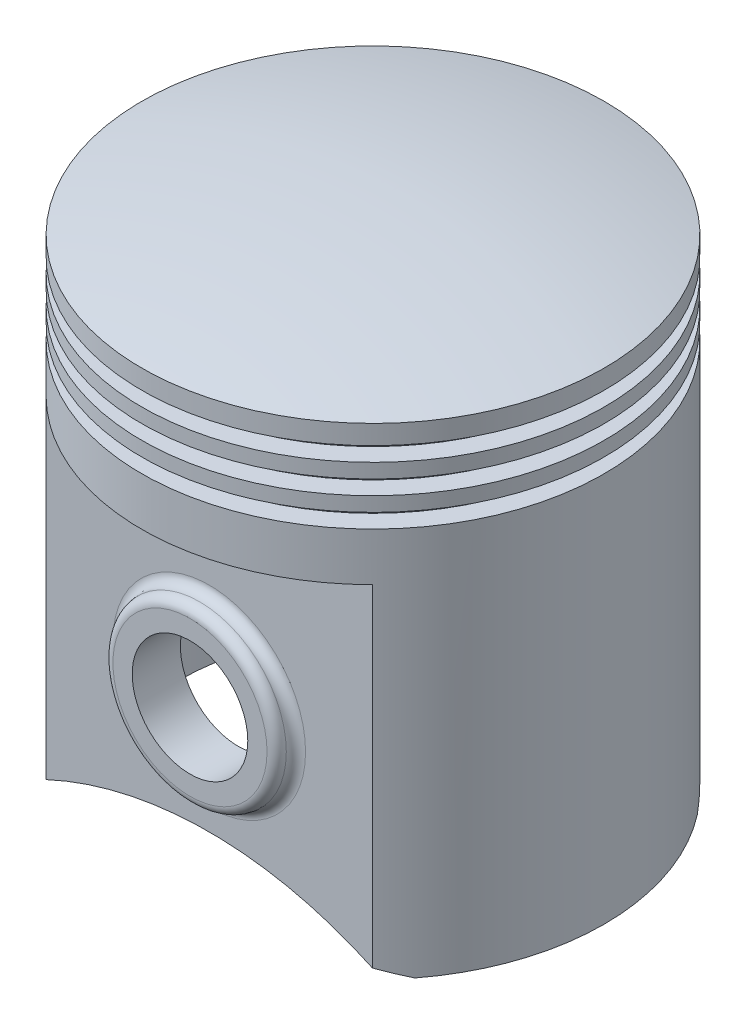
ISO-10303-21;
HEADER;
FILE_DESCRIPTION(('STEP AP214'),'2;1');
FILE_NAME('part.step','',(''),(''),'','','');
FILE_SCHEMA(('AUTOMOTIVE_DESIGN { 1 0 10303 214 1 1 1 1 }'));
ENDSEC;
DATA;
#1=APPLICATION_CONTEXT('core data for automotive mechanical design processes');
#2=APPLICATION_PROTOCOL_DEFINITION('international standard','automotive_design',2000,#1);
#3=PRODUCT_CONTEXT('',#1,'mechanical');
#4=PRODUCT('Part','Part','',(#3));
#5=PRODUCT_RELATED_PRODUCT_CATEGORY('part','',(#4));
#6=PRODUCT_DEFINITION_FORMATION('','',#4);
#7=PRODUCT_DEFINITION_CONTEXT('part definition',#1,'design');
#8=PRODUCT_DEFINITION('design','',#6,#7);
#9=PRODUCT_DEFINITION_SHAPE('','',#8);
#10=(LENGTH_UNIT() NAMED_UNIT(*) SI_UNIT(.MILLI.,.METRE.));
#11=(NAMED_UNIT(*) PLANE_ANGLE_UNIT() SI_UNIT($,.RADIAN.));
#12=(NAMED_UNIT(*) SI_UNIT($,.STERADIAN.) SOLID_ANGLE_UNIT());
#13=UNCERTAINTY_MEASURE_WITH_UNIT(LENGTH_MEASURE(1.E-05),#10,'distance_accuracy_value','');
#14=(GEOMETRIC_REPRESENTATION_CONTEXT(3) GLOBAL_UNCERTAINTY_ASSIGNED_CONTEXT((#13)) GLOBAL_UNIT_ASSIGNED_CONTEXT((#10,
#11,#12)) REPRESENTATION_CONTEXT('',''));
#15=CARTESIAN_POINT('',(0.,0.,0.));
#16=DIRECTION('',(0.,0.,1.));
#17=DIRECTION('',(1.,0.,0.));
#18=AXIS2_PLACEMENT_3D('',#15,#16,#17);
#19=CARTESIAN_POINT('',(0.,-35.1994318135961,-24.));
#20=DIRECTION('',(0.,0.,1.));
#21=DIRECTION('',(1.,0.,0.));
#22=AXIS2_PLACEMENT_3D('',#19,#20,#21);
#23=CYLINDRICAL_SURFACE('',#22,40.);
#24=CARTESIAN_POINT('',(19.,0.,14.6628782986152));
#25=CARTESIAN_POINT('',(18.5847844154625,0.22417514231841,15.2008416674184));
#26=CARTESIAN_POINT('',(18.1472749531916,0.450800853525988,15.720583924078));
#27=CARTESIAN_POINT('',(17.229430924885,0.903305358323858,16.7214980336072));
#28=CARTESIAN_POINT('',(16.7490810754239,1.12918385529891,17.2026560042297));
#29=CARTESIAN_POINT('',(15.7443796223877,1.57581717355902,18.1268646371823));
#30=CARTESIAN_POINT('',(15.2197634518151,1.79652939269345,18.5696486228512));
#31=CARTESIAN_POINT('',(14.1313833599364,2.22577453935094,19.4107434347561));
#32=CARTESIAN_POINT('',(13.5676231295076,2.43430861174211,19.8090584447426));
#33=CARTESIAN_POINT('',(12.4014963081478,2.83455429887705,20.5593059044338));
#34=CARTESIAN_POINT('',(11.7990100002299,3.02620893339201,20.9110831218259));
#35=CARTESIAN_POINT('',(10.5602218766716,3.3868064026951,21.5632002725983));
#36=CARTESIAN_POINT('',(9.92391895773195,3.55574849582937,21.8635385263817));
#37=CARTESIAN_POINT('',(8.62342320840555,3.86566866892299,22.4083047027535));
#38=CARTESIAN_POINT('',(7.95931483522713,4.00672490493522,22.6528891907548));
#39=CARTESIAN_POINT('',(6.60663592930378,4.25719223749272,23.0836725338871));
#40=CARTESIAN_POINT('',(5.91806903944259,4.36660802460178,23.2698800435048));
#41=CARTESIAN_POINT('',(4.59215338262825,4.54114914570338,23.5653660010413));
#42=CARTESIAN_POINT('',(3.95653429291983,4.60960046747166,23.6804595182362));
#43=CARTESIAN_POINT('',(2.67557620841154,4.71615638306671,23.8591567014349));
#44=CARTESIAN_POINT('',(2.03023785659978,4.75426297547383,23.9227637584713));
#45=CARTESIAN_POINT('',(0.735406969306551,4.79905416078167,23.9974950965044));
#46=CARTESIAN_POINT('',(0.0859142139936218,4.80573707688299,24.0086165768174));
#47=CARTESIAN_POINT('',(-1.21136844174268,4.78748235913691,23.9781873674946));
#48=CARTESIAN_POINT('',(-1.85915844199787,4.76254662247324,23.9366398381071));
#49=CARTESIAN_POINT('',(-3.08243340113651,4.68584919285358,23.8083586990923));
#50=CARTESIAN_POINT('',(-3.65863458605366,4.63703953335834,23.7265929391012));
#51=CARTESIAN_POINT('',(-4.80109464708866,4.51554548314267,23.5220364728596));
#52=CARTESIAN_POINT('',(-5.36735434428124,4.44286307395504,23.3992491715449));
#53=CARTESIAN_POINT('',(-6.48634583000771,4.27521075369698,23.114080016908));
#54=CARTESIAN_POINT('',(-7.03907894850286,4.18024304356482,22.9517020735703));
#55=CARTESIAN_POINT('',(-8.12798429480032,3.96998748429119,22.5890510227209));
#56=CARTESIAN_POINT('',(-8.66415582672125,3.85469878266769,22.3887763253839));
#57=CARTESIAN_POINT('',(-9.73722129991614,3.60136511760673,21.943940565358));
#58=CARTESIAN_POINT('',(-10.27337378466,3.46262375974749,21.6979896936735));
#59=CARTESIAN_POINT('',(-11.3225328531231,3.16848610713638,21.1694433586757));
#60=CARTESIAN_POINT('',(-11.8355382041687,3.01308892688204,20.8868459468909));
#61=CARTESIAN_POINT('',(-12.8366727755807,2.68852054240194,20.2869564707954));
#62=CARTESIAN_POINT('',(-13.3247872626694,2.51934133079035,19.9696441998403));
#63=CARTESIAN_POINT('',(-14.2741592843496,2.17039703659009,19.3024597608394));
#64=CARTESIAN_POINT('',(-14.7354193578949,1.9906329579918,18.9525906790344));
#65=CARTESIAN_POINT('',(-15.53843000618,1.66118701859229,18.2966765814725));
#66=CARTESIAN_POINT('',(-15.8853582872057,1.51285349768682,17.9962608691975));
#67=CARTESIAN_POINT('',(-16.5607191727584,1.21319010561359,17.376780524918));
#68=CARTESIAN_POINT('',(-16.8891537602792,1.06186055805686,17.0577178998414));
#69=CARTESIAN_POINT('',(-17.5260491906291,0.758343983174592,16.4026139472068));
#70=CARTESIAN_POINT('',(-17.8345646435942,0.606160662421761,16.0666239670156));
#71=CARTESIAN_POINT('',(-18.4320760770373,0.302273870423554,15.377465633861));
#72=CARTESIAN_POINT('',(-18.7210707877824,0.150570431002778,15.0242961660177));
#73=CARTESIAN_POINT('',(-19.,0.,14.6628782986152));
#74=B_SPLINE_CURVE_WITH_KNOTS('',3,(#24,#25,#26,#27,#28,#29,#30,#31,#32,#33,#34,#35,#36,#37,#38,
#39,#40,#41,#42,#43,#44,#45,#46,#47,#48,#49,#50,#51,#52,#53,#54,#55,#56,#57,#58,#59,#60,#61,#62,
#63,#64,#65,#66,#67,#68,#69,#70,#71,#72,#73),.UNSPECIFIED.,.F.,.F.,(4,2,2,2,2,2,2,2,2,2,2,2,2,2,
2,2,2,2,2,2,2,2,2,2,4),(0.,2.14619201814741,4.29315278252665,6.45400344697563,8.6146506416545,
10.7823323717961,12.9500848680932,15.1116728494894,17.2729402200685,19.218937601111,
21.1648068032574,23.1107798377901,25.0566361154919,26.8066791459319,28.5565769525621,
30.3063020086725,32.0561004846409,33.872158160539,35.6883124346079,37.5055295280586,
39.3225745325596,40.7687722984554,42.2148146987619,43.6567076951116,45.0986943897096),.UNSPECIFIED.);
#75=CARTESIAN_POINT('',(19.,0.,14.6628782986152));
#76=VERTEX_POINT('',#75);
#77=CARTESIAN_POINT('',(16.9410743460974,1.03591005039079,17.));
#78=VERTEX_POINT('',#77);
#79=EDGE_CURVE('E202',#76,#78,#74,.T.);
#80=ORIENTED_EDGE('',*,*,#79,.T.);
#81=CARTESIAN_POINT('',(0.,-35.1994318135961,17.));
#82=DIRECTION('',(0.,0.,-1.));
#83=DIRECTION('',(-1.,0.,0.));
#84=AXIS2_PLACEMENT_3D('',#81,#82,#83);
#85=CIRCLE('',#84,40.);
#86=CARTESIAN_POINT('',(-16.9410743460974,1.03591005039079,17.));
#87=VERTEX_POINT('',#86);
#88=EDGE_CURVE('E154',#78,#87,#85,.F.);
#89=ORIENTED_EDGE('',*,*,#88,.T.);
#90=CARTESIAN_POINT('',(-19.,0.,14.6628782986152));
#91=VERTEX_POINT('',#90);
#92=EDGE_CURVE('E153',#87,#91,#74,.T.);
#93=ORIENTED_EDGE('',*,*,#92,.T.);
#94=DIRECTION('',(0.,0.,1.));
#95=VECTOR('',#94,1.);
#96=CARTESIAN_POINT('',(-19.,0.,-24.));
#97=LINE('',#96,#95);
#98=CARTESIAN_POINT('',(-19.,0.,6.24499799839839));
#99=VERTEX_POINT('',#98);
#100=EDGE_CURVE('E291',#91,#99,#97,.F.);
#101=ORIENTED_EDGE('',*,*,#100,.T.);
#102=CARTESIAN_POINT('',(-19.,0.,6.24499799839837));
#103=CARTESIAN_POINT('',(-18.8202585353319,0.0969817128532858,6.79197210301841));
#104=CARTESIAN_POINT('',(-18.6174589709661,0.204714498288521,7.32924799218901));
#105=CARTESIAN_POINT('',(-18.1681410350363,0.437393377984401,8.38124634634524));
#106=CARTESIAN_POINT('',(-17.9216299338799,0.562336608913622,8.89597254422526));
#107=CARTESIAN_POINT('',(-17.3921059919807,0.822781911629741,9.89072900060968));
#108=CARTESIAN_POINT('',(-17.1098421840393,0.958049413971564,10.3712212939202));
#109=CARTESIAN_POINT('',(-16.5076269288855,1.23692809207039,11.3051661022802));
#110=CARTESIAN_POINT('',(-16.1876897852406,1.38053609073414,11.7586287818938));
#111=CARTESIAN_POINT('',(-15.6075875463034,1.63089351304631,12.5124400289307));
#112=CARTESIAN_POINT('',(-15.3560767786114,1.73659212557669,12.8198482567428));
#113=CARTESIAN_POINT('',(-14.8336181639409,1.94951117012887,13.4210039659551));
#114=CARTESIAN_POINT('',(-14.5625515542914,2.05673705236659,13.7146463148781));
#115=CARTESIAN_POINT('',(-14.2828568570857,2.16365157094273,14.));
#116=B_SPLINE_CURVE_WITH_KNOTS('',3,(#102,#103,#104,#105,#106,#107,#108,#109,#110,#111,#112,
#113,#114,#115),.UNSPECIFIED.,.F.,.F.,(4,2,2,2,2,2,4),(0.,1.75066829987974,3.50104568906382,
5.21944897719957,6.93720192412629,8.16959104224677,9.41022371268353),.UNSPECIFIED.);
#117=CARTESIAN_POINT('',(-14.2828568570857,2.16365157094273,14.));
#118=VERTEX_POINT('',#117);
#119=EDGE_CURVE('E413',#99,#118,#116,.T.);
#120=ORIENTED_EDGE('',*,*,#119,.T.);
#121=CARTESIAN_POINT('',(0.,-35.1994318135961,14.));
#122=DIRECTION('',(0.,0.,1.));
#123=DIRECTION('',(1.,0.,0.));
#124=AXIS2_PLACEMENT_3D('',#121,#122,#123);
#125=CIRCLE('',#124,40.);
#126=CARTESIAN_POINT('',(14.2828568570857,2.16365157094272,14.));
#127=VERTEX_POINT('',#126);
#128=EDGE_CURVE('E253',#118,#127,#125,.F.);
#129=ORIENTED_EDGE('',*,*,#128,.T.);
#130=CARTESIAN_POINT('',(14.2828568570857,2.16365157094272,14.));
#131=CARTESIAN_POINT('',(14.6775131687569,2.01280729699775,13.5973677537348));
#132=CARTESIAN_POINT('',(15.0550498418311,1.8612961791732,13.1781481636073));
#133=CARTESIAN_POINT('',(15.7741579232714,1.56097502677152,12.3083178308759));
#134=CARTESIAN_POINT('',(16.1156954030899,1.41216764779983,11.857678128264));
#135=CARTESIAN_POINT('',(16.7541220935511,1.12438631173865,10.9365144759754));
#136=CARTESIAN_POINT('',(17.0517449304083,0.98527811151048,10.4665411255795));
#137=CARTESIAN_POINT('',(17.6077757822892,0.717991544973343,9.50137374432842));
#138=CARTESIAN_POINT('',(17.8662123403,0.589805253334924,9.00619842497101));
#139=CARTESIAN_POINT('',(18.2746614216328,0.38249383567688,8.13621217368548));
#140=CARTESIAN_POINT('',(18.4346757038592,0.299740972735459,7.76692986093451));
#141=CARTESIAN_POINT('',(18.7337473919056,0.14282623615124,7.01509751919342));
#142=CARTESIAN_POINT('',(18.8726505382507,0.0687284369135807,6.63247280860509));
#143=CARTESIAN_POINT('',(19.,0.,6.2449979983984));
#144=B_SPLINE_CURVE_WITH_KNOTS('',3,(#130,#131,#132,#133,#134,#135,#136,#137,#138,#139,#140,
#141,#142,#143),.UNSPECIFIED.,.F.,.F.,(4,2,2,2,2,2,4),(0.,1.75046610713076,3.50256751449379,
5.22090157760208,6.93797794376393,8.1698351473774,9.41030051506601),.UNSPECIFIED.);
#145=CARTESIAN_POINT('',(19.,0.,6.2449979983984));
#146=VERTEX_POINT('',#145);
#147=EDGE_CURVE('E241',#127,#146,#144,.T.);
#148=ORIENTED_EDGE('',*,*,#147,.T.);
#149=DIRECTION('',(0.,0.,1.));
#150=VECTOR('',#149,1.);
#151=CARTESIAN_POINT('',(19.,0.,-24.));
#152=LINE('',#151,#150);
#153=EDGE_CURVE('E281',#146,#76,#152,.T.);
#154=ORIENTED_EDGE('',*,*,#153,.T.);
#155=EDGE_LOOP('',(#80,#89,#93,#101,#120,#129,#148,#154));
#156=FACE_BOUND('',#155,.T.);
#157=ADVANCED_FACE('F44',(#156),#23,.F.);
#158=CARTESIAN_POINT('',(0.,0.,0.));
#159=DIRECTION('',(0.,-1.,0.));
#160=DIRECTION('',(0.,0.,-1.));
#161=AXIS2_PLACEMENT_3D('',#158,#159,#160);
#162=PLANE('',#161);
#163=CARTESIAN_POINT('',(0.,0.,0.));
#164=DIRECTION('',(0.,-1.,0.));
#165=DIRECTION('',(0.,0.,-1.));
#166=AXIS2_PLACEMENT_3D('',#163,#164,#165);
#167=CIRCLE('',#166,20.);
#168=CARTESIAN_POINT('',(19.,0.,-6.2449979983984));
#169=VERTEX_POINT('',#168);
#170=EDGE_CURVE('E175',#169,#146,#167,.T.);
#171=ORIENTED_EDGE('',*,*,#170,.F.);
#172=CARTESIAN_POINT('',(19.,0.,-14.6628782986152));
#173=VERTEX_POINT('',#172);
#174=EDGE_CURVE('E315',#173,#169,#152,.T.);
#175=ORIENTED_EDGE('',*,*,#174,.F.);
#176=CARTESIAN_POINT('',(0.,0.,0.));
#177=DIRECTION('',(0.,-1.,0.));
#178=DIRECTION('',(0.,0.,-1.));
#179=AXIS2_PLACEMENT_3D('',#176,#177,#178);
#180=CIRCLE('',#179,24.);
#181=EDGE_CURVE('E289',#173,#76,#180,.T.);
#182=ORIENTED_EDGE('',*,*,#181,.T.);
#183=ORIENTED_EDGE('',*,*,#153,.F.);
#184=EDGE_LOOP('',(#171,#175,#182,#183));
#185=FACE_BOUND('',#184,.T.);
#186=ADVANCED_FACE('F275',(#185),#162,.T.);
#187=CARTESIAN_POINT('',(0.,-43.9999798630667,-0.0625025171167009));
#188=DIRECTION('',(-1.,0.,0.));
#189=DIRECTION('',(0.,0.,-1.));
#190=AXIS2_PLACEMENT_3D('',#187,#188,#189);
#191=CIRCLE('',#190,97.);
#192=TRIMMED_CURVE('',#191,(PARAMETER_VALUE(-1.57144068268605)),
(PARAMETER_VALUE(1.57144068268605)),.T.,.PARAMETER.);
#193=CARTESIAN_POINT('',(0.,-43.9999798630667,0.));
#194=DIRECTION('',(0.,-1.,0.));
#195=AXIS1_PLACEMENT('',#193,#194);
#196=SURFACE_OF_REVOLUTION('',#192,#195);
#197=CARTESIAN_POINT('',(0.,53.,0.));
#198=VERTEX_POINT('',#197);
#199=VERTEX_LOOP('',#198);
#200=FACE_BOUND('',#199,.T.);
#201=CARTESIAN_POINT('',(0.,50.,0.));
#202=DIRECTION('',(0.,-1.,0.));
#203=DIRECTION('',(0.,0.,-1.));
#204=AXIS2_PLACEMENT_3D('',#201,#202,#203);
#205=CIRCLE('',#204,24.);
#206=CARTESIAN_POINT('',(0.,50.,-24.));
#207=VERTEX_POINT('',#206);
#208=EDGE_CURVE('E308',#207,#207,#205,.T.);
#209=ORIENTED_EDGE('',*,*,#208,.F.);
#210=EDGE_LOOP('',(#209));
#211=FACE_BOUND('',#210,.T.);
#212=ADVANCED_FACE('F276',(#200,#211),#196,.T.);
#213=CARTESIAN_POINT('',(0.,0.,0.));
#214=DIRECTION('',(0.,-1.,0.));
#215=DIRECTION('',(0.,0.,-1.));
#216=AXIS2_PLACEMENT_3D('',#213,#214,#215);
#217=CYLINDRICAL_SURFACE('',#216,24.);
#218=ORIENTED_EDGE('',*,*,#208,.T.);
#219=EDGE_LOOP('',(#218));
#220=FACE_BOUND('',#219,.T.);
#221=CARTESIAN_POINT('',(0.,48.,0.));
#222=DIRECTION('',(0.,-1.,0.));
#223=DIRECTION('',(0.,0.,-1.));
#224=AXIS2_PLACEMENT_3D('',#221,#222,#223);
#225=CIRCLE('',#224,24.);
#226=CARTESIAN_POINT('',(0.,48.,-24.));
#227=VERTEX_POINT('',#226);
#228=EDGE_CURVE('E306',#227,#227,#225,.T.);
#229=ORIENTED_EDGE('',*,*,#228,.F.);
#230=EDGE_LOOP('',(#229));
#231=FACE_BOUND('',#230,.T.);
#232=ADVANCED_FACE('F356',(#220,#231),#217,.T.);
#233=CARTESIAN_POINT('',(22.,48.,0.));
#234=DIRECTION('',(0.,-1.,0.));
#235=DIRECTION('',(0.,0.,-1.));
#236=AXIS2_PLACEMENT_3D('',#233,#234,#235);
#237=PLANE('',#236);
#238=ORIENTED_EDGE('',*,*,#228,.T.);
#239=EDGE_LOOP('',(#238));
#240=FACE_BOUND('',#239,.T.);
#241=CARTESIAN_POINT('',(0.,48.,0.));
#242=DIRECTION('',(0.,-1.,0.));
#243=DIRECTION('',(0.,0.,-1.));
#244=AXIS2_PLACEMENT_3D('',#241,#242,#243);
#245=CIRCLE('',#244,22.);
#246=CARTESIAN_POINT('',(0.,48.,-22.));
#247=VERTEX_POINT('',#246);
#248=EDGE_CURVE('E348',#247,#247,#245,.T.);
#249=ORIENTED_EDGE('',*,*,#248,.F.);
#250=EDGE_LOOP('',(#249));
#251=FACE_BOUND('',#250,.T.);
#252=ADVANCED_FACE('F353',(#240,#251),#237,.T.);
#253=CARTESIAN_POINT('',(0.,0.,0.));
#254=DIRECTION('',(0.,-1.,0.));
#255=DIRECTION('',(0.,0.,-1.));
#256=AXIS2_PLACEMENT_3D('',#253,#254,#255);
#257=CYLINDRICAL_SURFACE('',#256,22.);
#258=ORIENTED_EDGE('',*,*,#248,.T.);
#259=EDGE_LOOP('',(#258));
#260=FACE_BOUND('',#259,.T.);
#261=CARTESIAN_POINT('',(0.,46.5,0.));
#262=DIRECTION('',(0.,-1.,0.));
#263=DIRECTION('',(0.,0.,-1.));
#264=AXIS2_PLACEMENT_3D('',#261,#262,#263);
#265=CIRCLE('',#264,22.);
#266=CARTESIAN_POINT('',(0.,46.5,-22.));
#267=VERTEX_POINT('',#266);
#268=EDGE_CURVE('E350',#267,#267,#265,.T.);
#269=ORIENTED_EDGE('',*,*,#268,.F.);
#270=EDGE_LOOP('',(#269));
#271=FACE_BOUND('',#270,.T.);
#272=ADVANCED_FACE('F368',(#260,#271),#257,.T.);
#273=CARTESIAN_POINT('',(24.,46.5,0.));
#274=DIRECTION('',(0.,1.,0.));
#275=DIRECTION('',(0.,0.,1.));
#276=AXIS2_PLACEMENT_3D('',#273,#274,#275);
#277=PLANE('',#276);
#278=ORIENTED_EDGE('',*,*,#268,.T.);
#279=EDGE_LOOP('',(#278));
#280=FACE_BOUND('',#279,.T.);
#281=CARTESIAN_POINT('',(0.,46.5,0.));
#282=DIRECTION('',(0.,-1.,0.));
#283=DIRECTION('',(0.,0.,-1.));
#284=AXIS2_PLACEMENT_3D('',#281,#282,#283);
#285=CIRCLE('',#284,24.);
#286=CARTESIAN_POINT('',(0.,46.5,-24.));
#287=VERTEX_POINT('',#286);
#288=EDGE_CURVE('E344',#287,#287,#285,.T.);
#289=ORIENTED_EDGE('',*,*,#288,.F.);
#290=EDGE_LOOP('',(#289));
#291=FACE_BOUND('',#290,.T.);
#292=ADVANCED_FACE('F677',(#280,#291),#277,.T.);
#293=CARTESIAN_POINT('',(0.,0.,0.));
#294=DIRECTION('',(0.,-1.,0.));
#295=DIRECTION('',(0.,0.,-1.));
#296=AXIS2_PLACEMENT_3D('',#293,#294,#295);
#297=CYLINDRICAL_SURFACE('',#296,24.);
#298=ORIENTED_EDGE('',*,*,#288,.T.);
#299=EDGE_LOOP('',(#298));
#300=FACE_BOUND('',#299,.T.);
#301=CARTESIAN_POINT('',(0.,45.,0.));
#302=DIRECTION('',(0.,-1.,0.));
#303=DIRECTION('',(0.,0.,-1.));
#304=AXIS2_PLACEMENT_3D('',#301,#302,#303);
#305=CIRCLE('',#304,24.);
#306=CARTESIAN_POINT('',(0.,45.,-24.));
#307=VERTEX_POINT('',#306);
#308=EDGE_CURVE('E343',#307,#307,#305,.T.);
#309=ORIENTED_EDGE('',*,*,#308,.F.);
#310=EDGE_LOOP('',(#309));
#311=FACE_BOUND('',#310,.T.);
#312=ADVANCED_FACE('F669',(#300,#311),#297,.T.);
#313=CARTESIAN_POINT('',(22.,45.,0.));
#314=DIRECTION('',(0.,-1.,0.));
#315=DIRECTION('',(0.,0.,-1.));
#316=AXIS2_PLACEMENT_3D('',#313,#314,#315);
#317=PLANE('',#316);
#318=ORIENTED_EDGE('',*,*,#308,.T.);
#319=EDGE_LOOP('',(#318));
#320=FACE_BOUND('',#319,.T.);
#321=CARTESIAN_POINT('',(0.,45.,0.));
#322=DIRECTION('',(0.,-1.,0.));
#323=DIRECTION('',(0.,0.,-1.));
#324=AXIS2_PLACEMENT_3D('',#321,#322,#323);
#325=CIRCLE('',#324,22.);
#326=CARTESIAN_POINT('',(0.,45.,-22.));
#327=VERTEX_POINT('',#326);
#328=EDGE_CURVE('E340',#327,#327,#325,.T.);
#329=ORIENTED_EDGE('',*,*,#328,.F.);
#330=EDGE_LOOP('',(#329));
#331=FACE_BOUND('',#330,.T.);
#332=ADVANCED_FACE('F660',(#320,#331),#317,.T.);
#333=CARTESIAN_POINT('',(0.,0.,0.));
#334=DIRECTION('',(0.,-1.,0.));
#335=DIRECTION('',(0.,0.,-1.));
#336=AXIS2_PLACEMENT_3D('',#333,#334,#335);
#337=CYLINDRICAL_SURFACE('',#336,22.);
#338=ORIENTED_EDGE('',*,*,#328,.T.);
#339=EDGE_LOOP('',(#338));
#340=FACE_BOUND('',#339,.T.);
#341=CARTESIAN_POINT('',(0.,43.5,0.));
#342=DIRECTION('',(0.,-1.,0.));
#343=DIRECTION('',(0.,0.,-1.));
#344=AXIS2_PLACEMENT_3D('',#341,#342,#343);
#345=CIRCLE('',#344,22.);
#346=CARTESIAN_POINT('',(0.,43.5,-22.));
#347=VERTEX_POINT('',#346);
#348=EDGE_CURVE('E333',#347,#347,#345,.T.);
#349=ORIENTED_EDGE('',*,*,#348,.F.);
#350=EDGE_LOOP('',(#349));
#351=FACE_BOUND('',#350,.T.);
#352=ADVANCED_FACE('F648',(#340,#351),#337,.T.);
#353=CARTESIAN_POINT('',(24.,43.5,0.));
#354=DIRECTION('',(0.,1.,0.));
#355=DIRECTION('',(0.,0.,1.));
#356=AXIS2_PLACEMENT_3D('',#353,#354,#355);
#357=PLANE('',#356);
#358=ORIENTED_EDGE('',*,*,#348,.T.);
#359=EDGE_LOOP('',(#358));
#360=FACE_BOUND('',#359,.T.);
#361=CARTESIAN_POINT('',(0.,43.5,0.));
#362=DIRECTION('',(0.,-1.,0.));
#363=DIRECTION('',(0.,0.,-1.));
#364=AXIS2_PLACEMENT_3D('',#361,#362,#363);
#365=CIRCLE('',#364,24.);
#366=CARTESIAN_POINT('',(0.,43.5,-24.));
#367=VERTEX_POINT('',#366);
#368=EDGE_CURVE('E335',#367,#367,#365,.T.);
#369=ORIENTED_EDGE('',*,*,#368,.F.);
#370=EDGE_LOOP('',(#369));
#371=FACE_BOUND('',#370,.T.);
#372=ADVANCED_FACE('F640',(#360,#371),#357,.T.);
#373=CARTESIAN_POINT('',(0.,0.,0.));
#374=DIRECTION('',(0.,-1.,0.));
#375=DIRECTION('',(0.,0.,-1.));
#376=AXIS2_PLACEMENT_3D('',#373,#374,#375);
#377=CYLINDRICAL_SURFACE('',#376,24.);
#378=ORIENTED_EDGE('',*,*,#368,.T.);
#379=EDGE_LOOP('',(#378));
#380=FACE_BOUND('',#379,.T.);
#381=CARTESIAN_POINT('',(0.,42.,0.));
#382=DIRECTION('',(0.,-1.,0.));
#383=DIRECTION('',(0.,0.,-1.));
#384=AXIS2_PLACEMENT_3D('',#381,#382,#383);
#385=CIRCLE('',#384,24.);
#386=CARTESIAN_POINT('',(0.,42.,-24.));
#387=VERTEX_POINT('',#386);
#388=EDGE_CURVE('E328',#387,#387,#385,.T.);
#389=ORIENTED_EDGE('',*,*,#388,.F.);
#390=EDGE_LOOP('',(#389));
#391=FACE_BOUND('',#390,.T.);
#392=ADVANCED_FACE('F628',(#380,#391),#377,.T.);
#393=CARTESIAN_POINT('',(22.,42.,0.));
#394=DIRECTION('',(0.,-1.,0.));
#395=DIRECTION('',(0.,0.,-1.));
#396=AXIS2_PLACEMENT_3D('',#393,#394,#395);
#397=PLANE('',#396);
#398=ORIENTED_EDGE('',*,*,#388,.T.);
#399=EDGE_LOOP('',(#398));
#400=FACE_BOUND('',#399,.T.);
#401=CARTESIAN_POINT('',(0.,42.,0.));
#402=DIRECTION('',(0.,-1.,0.));
#403=DIRECTION('',(0.,0.,-1.));
#404=AXIS2_PLACEMENT_3D('',#401,#402,#403);
#405=CIRCLE('',#404,22.);
#406=CARTESIAN_POINT('',(0.,42.,-22.));
#407=VERTEX_POINT('',#406);
#408=EDGE_CURVE('E326',#407,#407,#405,.T.);
#409=ORIENTED_EDGE('',*,*,#408,.F.);
#410=EDGE_LOOP('',(#409));
#411=FACE_BOUND('',#410,.T.);
#412=ADVANCED_FACE('F617',(#400,#411),#397,.T.);
#413=CARTESIAN_POINT('',(0.,0.,0.));
#414=DIRECTION('',(0.,-1.,0.));
#415=DIRECTION('',(0.,0.,-1.));
#416=AXIS2_PLACEMENT_3D('',#413,#414,#415);
#417=CYLINDRICAL_SURFACE('',#416,22.);
#418=ORIENTED_EDGE('',*,*,#408,.T.);
#419=EDGE_LOOP('',(#418));
#420=FACE_BOUND('',#419,.T.);
#421=CARTESIAN_POINT('',(0.,40.5,0.));
#422=DIRECTION('',(0.,-1.,0.));
#423=DIRECTION('',(0.,0.,-1.));
#424=AXIS2_PLACEMENT_3D('',#421,#422,#423);
#425=CIRCLE('',#424,22.);
#426=CARTESIAN_POINT('',(0.,40.5,-22.));
#427=VERTEX_POINT('',#426);
#428=EDGE_CURVE('E321',#427,#427,#425,.T.);
#429=ORIENTED_EDGE('',*,*,#428,.F.);
#430=EDGE_LOOP('',(#429));
#431=FACE_BOUND('',#430,.T.);
#432=ADVANCED_FACE('F615',(#420,#431),#417,.T.);
#433=CARTESIAN_POINT('',(24.,40.5,0.));
#434=DIRECTION('',(0.,1.,0.));
#435=DIRECTION('',(0.,0.,1.));
#436=AXIS2_PLACEMENT_3D('',#433,#434,#435);
#437=PLANE('',#436);
#438=ORIENTED_EDGE('',*,*,#428,.T.);
#439=EDGE_LOOP('',(#438));
#440=FACE_BOUND('',#439,.T.);
#441=CARTESIAN_POINT('',(0.,40.5,0.));
#442=DIRECTION('',(0.,-1.,0.));
#443=DIRECTION('',(0.,0.,-1.));
#444=AXIS2_PLACEMENT_3D('',#441,#442,#443);
#445=CIRCLE('',#444,24.);
#446=CARTESIAN_POINT('',(0.,40.5,-24.));
#447=VERTEX_POINT('',#446);
#448=EDGE_CURVE('E317',#447,#447,#445,.T.);
#449=ORIENTED_EDGE('',*,*,#448,.F.);
#450=EDGE_LOOP('',(#449));
#451=FACE_BOUND('',#450,.T.);
#452=ADVANCED_FACE('F610',(#440,#451),#437,.T.);
#453=CARTESIAN_POINT('',(0.,0.,0.));
#454=DIRECTION('',(0.,-1.,0.));
#455=DIRECTION('',(0.,0.,-1.));
#456=AXIS2_PLACEMENT_3D('',#453,#454,#455);
#457=CYLINDRICAL_SURFACE('',#456,24.);
#458=DIRECTION('',(0.,-1.,0.));
#459=VECTOR('',#458,1.);
#460=CARTESIAN_POINT('',(16.9410743460974,35.5,17.));
#461=LINE('',#460,#459);
#462=CARTESIAN_POINT('',(16.9410743460974,35.5,17.));
#463=VERTEX_POINT('',#462);
#464=EDGE_CURVE('E150',#463,#78,#461,.T.);
#465=ORIENTED_EDGE('',*,*,#464,.T.);
#466=ORIENTED_EDGE('',*,*,#79,.F.);
#467=ORIENTED_EDGE('',*,*,#181,.F.);
#468=CARTESIAN_POINT('',(-19.,0.,-14.6628782986152));
#469=CARTESIAN_POINT('',(-18.5847844154625,0.22417514231841,-15.2008416674184));
#470=CARTESIAN_POINT('',(-18.1472749531916,0.450800853525988,-15.720583924078));
#471=CARTESIAN_POINT('',(-17.229430924885,0.903305358323858,-16.7214980336072));
#472=CARTESIAN_POINT('',(-16.7490810754239,1.12918385529891,-17.2026560042297));
#473=CARTESIAN_POINT('',(-15.7443796223877,1.57581717355902,-18.1268646371823));
#474=CARTESIAN_POINT('',(-15.2197634518151,1.79652939269345,-18.5696486228512));
#475=CARTESIAN_POINT('',(-14.1313833599364,2.22577453935094,-19.4107434347561));
#476=CARTESIAN_POINT('',(-13.5676231295076,2.43430861174211,-19.8090584447426));
#477=CARTESIAN_POINT('',(-12.4014963081478,2.83455429887705,-20.5593059044338));
#478=CARTESIAN_POINT('',(-11.7990100002299,3.02620893339201,-20.9110831218259));
#479=CARTESIAN_POINT('',(-10.5602218766716,3.3868064026951,-21.5632002725983));
#480=CARTESIAN_POINT('',(-9.92391895773195,3.55574849582937,-21.8635385263817));
#481=CARTESIAN_POINT('',(-8.62342320840555,3.86566866892299,-22.4083047027535));
#482=CARTESIAN_POINT('',(-7.95931483522713,4.00672490493522,-22.6528891907548));
#483=CARTESIAN_POINT('',(-6.60663592930378,4.25719223749272,-23.0836725338871));
#484=CARTESIAN_POINT('',(-5.91806903944259,4.36660802460178,-23.2698800435048));
#485=CARTESIAN_POINT('',(-4.59215338262825,4.54114914570338,-23.5653660010413));
#486=CARTESIAN_POINT('',(-3.95653429291983,4.60960046747166,-23.6804595182362));
#487=CARTESIAN_POINT('',(-2.67557620841154,4.71615638306671,-23.8591567014349));
#488=CARTESIAN_POINT('',(-2.03023785659978,4.75426297547383,-23.9227637584713));
#489=CARTESIAN_POINT('',(-0.735406969306551,4.79905416078167,-23.9974950965044));
#490=CARTESIAN_POINT('',(-0.0859142139936218,4.80573707688299,-24.0086165768174));
#491=CARTESIAN_POINT('',(1.21136844174268,4.78748235913691,-23.9781873674946));
#492=CARTESIAN_POINT('',(1.85915844199787,4.76254662247324,-23.9366398381071));
#493=CARTESIAN_POINT('',(3.08243340113651,4.68584919285358,-23.8083586990923));
#494=CARTESIAN_POINT('',(3.65863458605366,4.63703953335834,-23.7265929391012));
#495=CARTESIAN_POINT('',(4.80109464708866,4.51554548314267,-23.5220364728596));
#496=CARTESIAN_POINT('',(5.36735434428124,4.44286307395504,-23.3992491715449));
#497=CARTESIAN_POINT('',(6.48634583000771,4.27521075369698,-23.114080016908));
#498=CARTESIAN_POINT('',(7.03907894850286,4.18024304356482,-22.9517020735703));
#499=CARTESIAN_POINT('',(8.12798429480032,3.96998748429119,-22.5890510227209));
#500=CARTESIAN_POINT('',(8.66415582672125,3.85469878266769,-22.3887763253839));
#501=CARTESIAN_POINT('',(9.73722129991614,3.60136511760673,-21.943940565358));
#502=CARTESIAN_POINT('',(10.27337378466,3.46262375974749,-21.6979896936735));
#503=CARTESIAN_POINT('',(11.3225328531231,3.16848610713638,-21.1694433586757));
#504=CARTESIAN_POINT('',(11.8355382041687,3.01308892688204,-20.8868459468909));
#505=CARTESIAN_POINT('',(12.8366727755807,2.68852054240194,-20.2869564707954));
#506=CARTESIAN_POINT('',(13.3247872626694,2.51934133079035,-19.9696441998403));
#507=CARTESIAN_POINT('',(14.2741592843496,2.17039703659009,-19.3024597608394));
#508=CARTESIAN_POINT('',(14.7354193578949,1.9906329579918,-18.9525906790344));
#509=CARTESIAN_POINT('',(15.53843000618,1.66118701859229,-18.2966765814725));
#510=CARTESIAN_POINT('',(15.8853582872057,1.51285349768682,-17.9962608691975));
#511=CARTESIAN_POINT('',(16.5607191727584,1.21319010561359,-17.376780524918));
#512=CARTESIAN_POINT('',(16.8891537602792,1.06186055805686,-17.0577178998414));
#513=CARTESIAN_POINT('',(17.5260491906291,0.758343983174592,-16.4026139472068));
#514=CARTESIAN_POINT('',(17.8345646435942,0.606160662421761,-16.0666239670156));
#515=CARTESIAN_POINT('',(18.4320760770373,0.302273870423554,-15.377465633861));
#516=CARTESIAN_POINT('',(18.7210707877824,0.150570431002778,-15.0242961660177));
#517=CARTESIAN_POINT('',(19.,0.,-14.6628782986152));
#518=B_SPLINE_CURVE_WITH_KNOTS('',3,(#468,#469,#470,#471,#472,#473,#474,#475,#476,#477,#478,
#479,#480,#481,#482,#483,#484,#485,#486,#487,#488,#489,#490,#491,#492,#493,#494,#495,#496,#497,
#498,#499,#500,#501,#502,#503,#504,#505,#506,#507,#508,#509,#510,#511,#512,#513,#514,#515,#516,
#517),.UNSPECIFIED.,.F.,.F.,(4,2,2,2,2,2,2,2,2,2,2,2,2,2,2,2,2,2,2,2,2,2,2,2,4),(0.,
2.14619201814741,4.29315278252665,6.45400344697563,8.6146506416545,10.7823323717961,
12.9500848680932,15.1116728494894,17.2729402200685,19.218937601111,21.1648068032574,
23.1107798377901,25.0566361154919,26.8066791459319,28.5565769525621,30.3063020086725,
32.0561004846409,33.872158160539,35.6883124346079,37.5055295280586,39.3225745325596,
40.7687722984554,42.2148146987619,43.6567076951116,45.0986943897096),.UNSPECIFIED.);
#519=CARTESIAN_POINT('',(16.9410743460974,1.03591005039079,-17.));
#520=VERTEX_POINT('',#519);
#521=EDGE_CURVE('E190',#520,#173,#518,.T.);
#522=ORIENTED_EDGE('',*,*,#521,.F.);
#523=DIRECTION('',(0.,-1.,0.));
#524=VECTOR('',#523,1.);
#525=CARTESIAN_POINT('',(16.9410743460974,35.5,-17.));
#526=LINE('',#525,#524);
#527=CARTESIAN_POINT('',(16.9410743460974,35.5,-17.));
#528=VERTEX_POINT('',#527);
#529=EDGE_CURVE('E70',#528,#520,#526,.T.);
#530=ORIENTED_EDGE('',*,*,#529,.F.);
#531=CARTESIAN_POINT('',(0.,35.5,0.));
#532=DIRECTION('',(0.,-1.,0.));
#533=DIRECTION('',(0.,0.,-1.));
#534=AXIS2_PLACEMENT_3D('',#531,#532,#533);
#535=CIRCLE('',#534,24.);
#536=CARTESIAN_POINT('',(-16.9410743460974,35.5,-17.));
#537=VERTEX_POINT('',#536);
#538=EDGE_CURVE('E158',#537,#528,#535,.T.);
#539=ORIENTED_EDGE('',*,*,#538,.F.);
#540=DIRECTION('',(0.,-1.,0.));
#541=VECTOR('',#540,1.);
#542=CARTESIAN_POINT('',(-16.9410743460974,35.5,-17.));
#543=LINE('',#542,#541);
#544=CARTESIAN_POINT('',(-16.9410743460974,1.03591005039078,-17.));
#545=VERTEX_POINT('',#544);
#546=EDGE_CURVE('E143',#537,#545,#543,.T.);
#547=ORIENTED_EDGE('',*,*,#546,.T.);
#548=CARTESIAN_POINT('',(-19.,0.,-14.6628782986152));
#549=VERTEX_POINT('',#548);
#550=EDGE_CURVE('E198',#549,#545,#518,.T.);
#551=ORIENTED_EDGE('',*,*,#550,.F.);
#552=EDGE_CURVE('E290',#91,#549,#180,.T.);
#553=ORIENTED_EDGE('',*,*,#552,.F.);
#554=ORIENTED_EDGE('',*,*,#92,.F.);
#555=DIRECTION('',(0.,-1.,0.));
#556=VECTOR('',#555,1.);
#557=CARTESIAN_POINT('',(-16.9410743460974,35.5,17.));
#558=LINE('',#557,#556);
#559=CARTESIAN_POINT('',(-16.9410743460974,35.5,17.));
#560=VERTEX_POINT('',#559);
#561=EDGE_CURVE('E144',#560,#87,#558,.T.);
#562=ORIENTED_EDGE('',*,*,#561,.F.);
#563=CARTESIAN_POINT('',(0.,35.5,0.));
#564=DIRECTION('',(0.,-1.,0.));
#565=DIRECTION('',(0.,0.,-1.));
#566=AXIS2_PLACEMENT_3D('',#563,#564,#565);
#567=CIRCLE('',#566,24.);
#568=EDGE_CURVE('E138',#463,#560,#567,.T.);
#569=ORIENTED_EDGE('',*,*,#568,.F.);
#570=EDGE_LOOP('',(#465,#466,#467,#522,#530,#539,#547,#551,#553,#554,#562,#569));
#571=FACE_BOUND('',#570,.T.);
#572=ORIENTED_EDGE('',*,*,#448,.T.);
#573=EDGE_LOOP('',(#572));
#574=FACE_BOUND('',#573,.T.);
#575=ADVANCED_FACE('F147',(#571,#574),#457,.T.);
#576=CARTESIAN_POINT('',(0.,0.,0.));
#577=DIRECTION('',(0.,-1.,0.));
#578=DIRECTION('',(0.,0.,-1.));
#579=AXIS2_PLACEMENT_3D('',#576,#577,#578);
#580=CIRCLE('',#579,20.);
#581=CARTESIAN_POINT('',(-19.,0.,-6.24499799839839));
#582=VERTEX_POINT('',#581);
#583=EDGE_CURVE('E169',#99,#582,#580,.T.);
#584=ORIENTED_EDGE('',*,*,#583,.F.);
#585=ORIENTED_EDGE('',*,*,#100,.F.);
#586=ORIENTED_EDGE('',*,*,#552,.T.);
#587=EDGE_CURVE('E299',#582,#549,#97,.F.);
#588=ORIENTED_EDGE('',*,*,#587,.F.);
#589=EDGE_LOOP('',(#584,#585,#586,#588));
#590=FACE_BOUND('',#589,.T.);
#591=ADVANCED_FACE('F218',(#590),#162,.T.);
#592=ORIENTED_EDGE('',*,*,#550,.T.);
#593=CARTESIAN_POINT('',(0.,-35.1994318135961,-17.));
#594=DIRECTION('',(0.,0.,1.));
#595=DIRECTION('',(1.,0.,0.));
#596=AXIS2_PLACEMENT_3D('',#593,#594,#595);
#597=CIRCLE('',#596,40.);
#598=EDGE_CURVE('E303',#545,#520,#597,.F.);
#599=ORIENTED_EDGE('',*,*,#598,.T.);
#600=ORIENTED_EDGE('',*,*,#521,.T.);
#601=ORIENTED_EDGE('',*,*,#174,.T.);
#602=CARTESIAN_POINT('',(19.,0.,-6.24499799839839));
#603=CARTESIAN_POINT('',(18.8202585353319,0.0969817128532905,-6.79197210301843));
#604=CARTESIAN_POINT('',(18.6174589709661,0.204714498288526,-7.32924799218904));
#605=CARTESIAN_POINT('',(18.1681410350362,0.437393377984406,-8.38124634634527));
#606=CARTESIAN_POINT('',(17.9216299338799,0.562336608913628,-8.89597254422529));
#607=CARTESIAN_POINT('',(17.3921059919807,0.822781911629745,-9.89072900060971));
#608=CARTESIAN_POINT('',(17.1098421840393,0.958049413971565,-10.3712212939202));
#609=CARTESIAN_POINT('',(16.5076269288855,1.23692809207039,-11.3051661022802));
#610=CARTESIAN_POINT('',(16.1876897852405,1.38053609073414,-11.7586287818938));
#611=CARTESIAN_POINT('',(15.6075875463034,1.63089351304631,-12.5124400289307));
#612=CARTESIAN_POINT('',(15.3560767786114,1.73659212557669,-12.8198482567429));
#613=CARTESIAN_POINT('',(14.8336181639409,1.94951117012887,-13.4210039659552));
#614=CARTESIAN_POINT('',(14.5625515542914,2.05673705236659,-13.7146463148781));
#615=CARTESIAN_POINT('',(14.2828568570857,2.16365157094273,-14.));
#616=B_SPLINE_CURVE_WITH_KNOTS('',3,(#602,#603,#604,#605,#606,#607,#608,#609,#610,#611,#612,
#613,#614,#615),.UNSPECIFIED.,.F.,.F.,(4,2,2,2,2,2,4),(0.,1.75066829987974,3.50104568906383,
5.21944897719958,6.9372019241263,8.16959104224676,9.4102237126835),.UNSPECIFIED.);
#617=CARTESIAN_POINT('',(14.2828568570857,2.16365157094273,-14.));
#618=VERTEX_POINT('',#617);
#619=EDGE_CURVE('E228',#169,#618,#616,.T.);
#620=ORIENTED_EDGE('',*,*,#619,.T.);
#621=CARTESIAN_POINT('',(0.,-35.1994318135961,-14.));
#622=DIRECTION('',(0.,0.,-1.));
#623=DIRECTION('',(-1.,0.,0.));
#624=AXIS2_PLACEMENT_3D('',#621,#622,#623);
#625=CIRCLE('',#624,40.);
#626=CARTESIAN_POINT('',(-14.2828568570857,2.16365157094273,-14.));
#627=VERTEX_POINT('',#626);
#628=EDGE_CURVE('E314',#618,#627,#625,.F.);
#629=ORIENTED_EDGE('',*,*,#628,.T.);
#630=CARTESIAN_POINT('',(-14.2828568570857,2.16365157094272,-14.));
#631=CARTESIAN_POINT('',(-14.6775131687569,2.01280729699775,-13.5973677537348));
#632=CARTESIAN_POINT('',(-15.0550498418311,1.8612961791732,-13.1781481636073));
#633=CARTESIAN_POINT('',(-15.7741579232714,1.56097502677152,-12.3083178308759));
#634=CARTESIAN_POINT('',(-16.1156954030899,1.41216764779983,-11.857678128264));
#635=CARTESIAN_POINT('',(-16.7541220935511,1.12438631173866,-10.9365144759754));
#636=CARTESIAN_POINT('',(-17.0517449304083,0.985278111510485,-10.4665411255795));
#637=CARTESIAN_POINT('',(-17.6077757822892,0.717991544973348,-9.50137374432841));
#638=CARTESIAN_POINT('',(-17.8662123403,0.589805253334924,-9.006198424971));
#639=CARTESIAN_POINT('',(-18.2746614216328,0.38249383567688,-8.13621217368547));
#640=CARTESIAN_POINT('',(-18.4346757038592,0.299740972735462,-7.7669298609345));
#641=CARTESIAN_POINT('',(-18.7337473919056,0.142826236151246,-7.01509751919341));
#642=CARTESIAN_POINT('',(-18.8726505382507,0.068728436913587,-6.63247280860507));
#643=CARTESIAN_POINT('',(-19.,0.,-6.24499799839838));
#644=B_SPLINE_CURVE_WITH_KNOTS('',3,(#630,#631,#632,#633,#634,#635,#636,#637,#638,#639,#640,
#641,#642,#643),.UNSPECIFIED.,.F.,.F.,(4,2,2,2,2,2,4),(0.,1.75046610713076,3.50256751449379,
5.22090157760208,6.93797794376393,8.16983514737741,9.41030051506602),.UNSPECIFIED.);
#645=EDGE_CURVE('E236',#627,#582,#644,.T.);
#646=ORIENTED_EDGE('',*,*,#645,.T.);
#647=ORIENTED_EDGE('',*,*,#587,.T.);
#648=EDGE_LOOP('',(#592,#599,#600,#601,#620,#629,#646,#647));
#649=FACE_BOUND('',#648,.T.);
#650=ADVANCED_FACE('F212',(#649),#23,.F.);
#651=CARTESIAN_POINT('',(0.,37.,0.));
#652=DIRECTION('',(0.,-1.,0.));
#653=DIRECTION('',(0.,0.,-1.));
#654=AXIS2_PLACEMENT_3D('',#651,#652,#653);
#655=CYLINDRICAL_SURFACE('',#654,20.);
#656=ORIENTED_EDGE('',*,*,#583,.T.);
#657=ORIENTED_EDGE('',*,*,#645,.F.);
#658=DIRECTION('',(0.,-1.,0.));
#659=VECTOR('',#658,1.);
#660=CARTESIAN_POINT('',(-14.2828568570857,37.,-14.));
#661=LINE('',#660,#659);
#662=CARTESIAN_POINT('',(-14.2828568570857,37.,-14.));
#663=VERTEX_POINT('',#662);
#664=EDGE_CURVE('E185',#663,#627,#661,.T.);
#665=ORIENTED_EDGE('',*,*,#664,.F.);
#666=CARTESIAN_POINT('',(0.,37.,0.));
#667=DIRECTION('',(0.,-1.,0.));
#668=DIRECTION('',(0.,0.,-1.));
#669=AXIS2_PLACEMENT_3D('',#666,#667,#668);
#670=CIRCLE('',#669,20.);
#671=CARTESIAN_POINT('',(-14.2828568570857,37.,14.));
#672=VERTEX_POINT('',#671);
#673=EDGE_CURVE('E166',#672,#663,#670,.T.);
#674=ORIENTED_EDGE('',*,*,#673,.F.);
#675=DIRECTION('',(0.,-1.,0.));
#676=VECTOR('',#675,1.);
#677=CARTESIAN_POINT('',(-14.2828568570857,37.,14.));
#678=LINE('',#677,#676);
#679=EDGE_CURVE('E183',#672,#118,#678,.T.);
#680=ORIENTED_EDGE('',*,*,#679,.T.);
#681=ORIENTED_EDGE('',*,*,#119,.F.);
#682=EDGE_LOOP('',(#656,#657,#665,#674,#680,#681));
#683=FACE_BOUND('',#682,.T.);
#684=ADVANCED_FACE('F217',(#683),#655,.F.);
#685=CARTESIAN_POINT('',(-14.2828568570857,37.,14.));
#686=DIRECTION('',(0.,0.,1.));
#687=DIRECTION('',(1.,0.,0.));
#688=AXIS2_PLACEMENT_3D('',#685,#686,#687);
#689=PLANE('',#688);
#690=CARTESIAN_POINT('',(0.,17.,14.));
#691=DIRECTION('',(0.,0.,1.));
#692=DIRECTION('',(1.,0.,0.));
#693=AXIS2_PLACEMENT_3D('',#690,#691,#692);
#694=CIRCLE('',#693,6.);
#695=CARTESIAN_POINT('',(6.,17.,14.));
#696=VERTEX_POINT('',#695);
#697=EDGE_CURVE('E391',#696,#696,#694,.F.);
#698=ORIENTED_EDGE('',*,*,#697,.F.);
#699=EDGE_LOOP('',(#698));
#700=FACE_BOUND('',#699,.T.);
#701=ORIENTED_EDGE('',*,*,#679,.F.);
#702=DIRECTION('',(-1.,0.,0.));
#703=VECTOR('',#702,1.);
#704=CARTESIAN_POINT('',(-14.2828568570857,37.,14.));
#705=LINE('',#704,#703);
#706=CARTESIAN_POINT('',(14.2828568570857,37.,14.));
#707=VERTEX_POINT('',#706);
#708=EDGE_CURVE('E179',#707,#672,#705,.T.);
#709=ORIENTED_EDGE('',*,*,#708,.F.);
#710=DIRECTION('',(0.,-1.,0.));
#711=VECTOR('',#710,1.);
#712=CARTESIAN_POINT('',(14.2828568570857,37.,14.));
#713=LINE('',#712,#711);
#714=EDGE_CURVE('E186',#707,#127,#713,.T.);
#715=ORIENTED_EDGE('',*,*,#714,.T.);
#716=ORIENTED_EDGE('',*,*,#128,.F.);
#717=EDGE_LOOP('',(#701,#709,#715,#716));
#718=FACE_BOUND('',#717,.T.);
#719=ADVANCED_FACE('F260',(#700,#718),#689,.F.);
#720=CARTESIAN_POINT('',(0.,37.,0.));
#721=DIRECTION('',(0.,-1.,0.));
#722=DIRECTION('',(0.,0.,-1.));
#723=AXIS2_PLACEMENT_3D('',#720,#721,#722);
#724=CYLINDRICAL_SURFACE('',#723,20.);
#725=ORIENTED_EDGE('',*,*,#170,.T.);
#726=ORIENTED_EDGE('',*,*,#147,.F.);
#727=ORIENTED_EDGE('',*,*,#714,.F.);
#728=CARTESIAN_POINT('',(0.,37.,0.));
#729=DIRECTION('',(0.,-1.,0.));
#730=DIRECTION('',(0.,0.,-1.));
#731=AXIS2_PLACEMENT_3D('',#728,#729,#730);
#732=CIRCLE('',#731,20.);
#733=CARTESIAN_POINT('',(14.2828568570857,37.,-14.));
#734=VERTEX_POINT('',#733);
#735=EDGE_CURVE('E178',#734,#707,#732,.T.);
#736=ORIENTED_EDGE('',*,*,#735,.F.);
#737=DIRECTION('',(0.,-1.,0.));
#738=VECTOR('',#737,1.);
#739=CARTESIAN_POINT('',(14.2828568570857,37.,-14.));
#740=LINE('',#739,#738);
#741=EDGE_CURVE('E195',#734,#618,#740,.T.);
#742=ORIENTED_EDGE('',*,*,#741,.T.);
#743=ORIENTED_EDGE('',*,*,#619,.F.);
#744=EDGE_LOOP('',(#725,#726,#727,#736,#742,#743));
#745=FACE_BOUND('',#744,.T.);
#746=ADVANCED_FACE('F252',(#745),#724,.F.);
#747=CARTESIAN_POINT('',(-14.2828568570857,37.,-14.));
#748=DIRECTION('',(0.,0.,-1.));
#749=DIRECTION('',(-1.,0.,0.));
#750=AXIS2_PLACEMENT_3D('',#747,#748,#749);
#751=PLANE('',#750);
#752=CARTESIAN_POINT('',(0.,17.,-14.));
#753=DIRECTION('',(0.,0.,-1.));
#754=DIRECTION('',(-1.,0.,0.));
#755=AXIS2_PLACEMENT_3D('',#752,#753,#754);
#756=CIRCLE('',#755,6.);
#757=CARTESIAN_POINT('',(-6.,17.,-14.));
#758=VERTEX_POINT('',#757);
#759=EDGE_CURVE('E771',#758,#758,#756,.T.);
#760=ORIENTED_EDGE('',*,*,#759,.T.);
#761=EDGE_LOOP('',(#760));
#762=FACE_BOUND('',#761,.T.);
#763=ORIENTED_EDGE('',*,*,#741,.F.);
#764=DIRECTION('',(1.,0.,0.));
#765=VECTOR('',#764,1.);
#766=CARTESIAN_POINT('',(-14.2828568570857,37.,-14.));
#767=LINE('',#766,#765);
#768=EDGE_CURVE('E174',#663,#734,#767,.T.);
#769=ORIENTED_EDGE('',*,*,#768,.F.);
#770=ORIENTED_EDGE('',*,*,#664,.T.);
#771=ORIENTED_EDGE('',*,*,#628,.F.);
#772=EDGE_LOOP('',(#763,#769,#770,#771));
#773=FACE_BOUND('',#772,.T.);
#774=ADVANCED_FACE('F258',(#762,#773),#751,.F.);
#775=CARTESIAN_POINT('',(0.,37.,0.));
#776=DIRECTION('',(0.,-1.,0.));
#777=DIRECTION('',(0.,0.,-1.));
#778=AXIS2_PLACEMENT_3D('',#775,#776,#777);
#779=PLANE('',#778);
#780=ORIENTED_EDGE('',*,*,#673,.T.);
#781=ORIENTED_EDGE('',*,*,#768,.T.);
#782=ORIENTED_EDGE('',*,*,#735,.T.);
#783=ORIENTED_EDGE('',*,*,#708,.T.);
#784=EDGE_LOOP('',(#780,#781,#782,#783));
#785=FACE_BOUND('',#784,.T.);
#786=ADVANCED_FACE('F265',(#785),#779,.T.);
#787=CARTESIAN_POINT('',(-16.9410743460974,35.5,-17.));
#788=DIRECTION('',(0.,0.,1.));
#789=DIRECTION('',(1.,0.,0.));
#790=AXIS2_PLACEMENT_3D('',#787,#788,#789);
#791=PLANE('',#790);
#792=CARTESIAN_POINT('',(0.,17.,-17.));
#793=DIRECTION('',(0.,0.,1.));
#794=DIRECTION('',(1.,0.,0.));
#795=AXIS2_PLACEMENT_3D('',#792,#793,#794);
#796=CIRCLE('',#795,9.);
#797=CARTESIAN_POINT('',(9.,17.,-17.));
#798=VERTEX_POINT('',#797);
#799=EDGE_CURVE('E399',#798,#798,#796,.T.);
#800=ORIENTED_EDGE('',*,*,#799,.T.);
#801=EDGE_LOOP('',(#800));
#802=FACE_BOUND('',#801,.T.);
#803=ORIENTED_EDGE('',*,*,#546,.F.);
#804=DIRECTION('',(-1.,0.,0.));
#805=VECTOR('',#804,1.);
#806=CARTESIAN_POINT('',(-16.9410743460974,35.5,-17.));
#807=LINE('',#806,#805);
#808=EDGE_CURVE('E159',#528,#537,#807,.T.);
#809=ORIENTED_EDGE('',*,*,#808,.F.);
#810=ORIENTED_EDGE('',*,*,#529,.T.);
#811=ORIENTED_EDGE('',*,*,#598,.F.);
#812=EDGE_LOOP('',(#803,#809,#810,#811));
#813=FACE_BOUND('',#812,.T.);
#814=ADVANCED_FACE('F270',(#802,#813),#791,.F.);
#815=CARTESIAN_POINT('',(0.,35.5,0.));
#816=DIRECTION('',(0.,-1.,0.));
#817=DIRECTION('',(0.,0.,-1.));
#818=AXIS2_PLACEMENT_3D('',#815,#816,#817);
#819=PLANE('',#818);
#820=ORIENTED_EDGE('',*,*,#538,.T.);
#821=ORIENTED_EDGE('',*,*,#808,.T.);
#822=EDGE_LOOP('',(#820,#821));
#823=FACE_BOUND('',#822,.T.);
#824=ADVANCED_FACE('F541',(#823),#819,.T.);
#825=CARTESIAN_POINT('',(-16.9410743460974,35.5,17.));
#826=DIRECTION('',(0.,0.,-1.));
#827=DIRECTION('',(-1.,0.,0.));
#828=AXIS2_PLACEMENT_3D('',#825,#826,#827);
#829=PLANE('',#828);
#830=CARTESIAN_POINT('',(0.,17.,17.));
#831=DIRECTION('',(0.,0.,-1.));
#832=DIRECTION('',(-1.,0.,0.));
#833=AXIS2_PLACEMENT_3D('',#830,#831,#832);
#834=CIRCLE('',#833,10.);
#835=CARTESIAN_POINT('',(-10.,17.,17.));
#836=VERTEX_POINT('',#835);
#837=EDGE_CURVE('E388',#836,#836,#834,.T.);
#838=ORIENTED_EDGE('',*,*,#837,.T.);
#839=EDGE_LOOP('',(#838));
#840=FACE_BOUND('',#839,.T.);
#841=ORIENTED_EDGE('',*,*,#464,.F.);
#842=DIRECTION('',(1.,0.,0.));
#843=VECTOR('',#842,1.);
#844=CARTESIAN_POINT('',(-16.9410743460974,35.5,17.));
#845=LINE('',#844,#843);
#846=EDGE_CURVE('E56',#560,#463,#845,.T.);
#847=ORIENTED_EDGE('',*,*,#846,.F.);
#848=ORIENTED_EDGE('',*,*,#561,.T.);
#849=ORIENTED_EDGE('',*,*,#88,.F.);
#850=EDGE_LOOP('',(#841,#847,#848,#849));
#851=FACE_BOUND('',#850,.T.);
#852=ADVANCED_FACE('F145',(#840,#851),#829,.F.);
#853=CARTESIAN_POINT('',(0.,35.5,0.));
#854=DIRECTION('',(0.,-1.,0.));
#855=DIRECTION('',(0.,0.,-1.));
#856=AXIS2_PLACEMENT_3D('',#853,#854,#855);
#857=PLANE('',#856);
#858=ORIENTED_EDGE('',*,*,#568,.T.);
#859=ORIENTED_EDGE('',*,*,#846,.T.);
#860=EDGE_LOOP('',(#858,#859));
#861=FACE_BOUND('',#860,.T.);
#862=ADVANCED_FACE('F140',(#861),#857,.T.);
#863=CARTESIAN_POINT('',(0.,17.,19.));
#864=DIRECTION('',(0.,0.,1.));
#865=DIRECTION('',(1.,0.,0.));
#866=AXIS2_PLACEMENT_3D('',#863,#864,#865);
#867=PLANE('',#866);
#868=CARTESIAN_POINT('',(0.,17.,19.));
#869=DIRECTION('',(0.,0.,1.));
#870=DIRECTION('',(1.,0.,0.));
#871=AXIS2_PLACEMENT_3D('',#868,#869,#870);
#872=CIRCLE('',#871,8.);
#873=CARTESIAN_POINT('',(8.,17.,19.));
#874=VERTEX_POINT('',#873);
#875=EDGE_CURVE('E407',#874,#874,#872,.T.);
#876=ORIENTED_EDGE('',*,*,#875,.T.);
#877=EDGE_LOOP('',(#876));
#878=FACE_BOUND('',#877,.T.);
#879=CARTESIAN_POINT('',(0.,17.,19.));
#880=DIRECTION('',(0.,0.,1.));
#881=DIRECTION('',(1.,0.,0.));
#882=AXIS2_PLACEMENT_3D('',#879,#880,#881);
#883=CIRCLE('',#882,6.);
#884=CARTESIAN_POINT('',(6.,17.,19.));
#885=VERTEX_POINT('',#884);
#886=EDGE_CURVE('E161',#885,#885,#883,.T.);
#887=ORIENTED_EDGE('',*,*,#886,.F.);
#888=EDGE_LOOP('',(#887));
#889=FACE_BOUND('',#888,.T.);
#890=ADVANCED_FACE('F383',(#878,#889),#867,.T.);
#891=CARTESIAN_POINT('',(0.,17.,19.));
#892=DIRECTION('',(0.,0.,-1.));
#893=DIRECTION('',(-1.,0.,0.));
#894=AXIS2_PLACEMENT_3D('',#891,#892,#893);
#895=CYLINDRICAL_SURFACE('',#894,6.);
#896=ORIENTED_EDGE('',*,*,#886,.T.);
#897=EDGE_LOOP('',(#896));
#898=FACE_BOUND('',#897,.T.);
#899=ORIENTED_EDGE('',*,*,#697,.T.);
#900=EDGE_LOOP('',(#899));
#901=FACE_BOUND('',#900,.T.);
#902=ADVANCED_FACE('F378',(#898,#901),#895,.F.);
#903=CARTESIAN_POINT('',(0.,17.,18.));
#904=DIRECTION('',(0.,0.,-1.));
#905=DIRECTION('',(-1.,0.,0.));
#906=AXIS2_PLACEMENT_3D('',#903,#904,#905);
#907=TOROIDAL_SURFACE('',#906,10.,1.);
#908=ORIENTED_EDGE('',*,*,#837,.F.);
#909=EDGE_LOOP('',(#908));
#910=FACE_BOUND('',#909,.T.);
#911=CARTESIAN_POINT('',(0.,17.,18.));
#912=DIRECTION('',(0.,0.,-1.));
#913=DIRECTION('',(-1.,0.,0.));
#914=AXIS2_PLACEMENT_3D('',#911,#912,#913);
#915=CIRCLE('',#914,9.);
#916=CARTESIAN_POINT('',(-9.,17.,18.));
#917=VERTEX_POINT('',#916);
#918=EDGE_CURVE('E395',#917,#917,#915,.F.);
#919=ORIENTED_EDGE('',*,*,#918,.F.);
#920=EDGE_LOOP('',(#919));
#921=FACE_BOUND('',#920,.T.);
#922=ADVANCED_FACE('F374',(#910,#921),#907,.F.);
#923=CARTESIAN_POINT('',(0.,17.,18.));
#924=DIRECTION('',(0.,0.,1.));
#925=DIRECTION('',(1.,0.,0.));
#926=AXIS2_PLACEMENT_3D('',#923,#924,#925);
#927=TOROIDAL_SURFACE('',#926,8.,1.);
#928=ORIENTED_EDGE('',*,*,#918,.T.);
#929=EDGE_LOOP('',(#928));
#930=FACE_BOUND('',#929,.T.);
#931=ORIENTED_EDGE('',*,*,#875,.F.);
#932=EDGE_LOOP('',(#931));
#933=FACE_BOUND('',#932,.T.);
#934=ADVANCED_FACE('F375',(#930,#933),#927,.T.);
#935=CARTESIAN_POINT('',(0.,17.,-19.));
#936=DIRECTION('',(0.,0.,1.));
#937=DIRECTION('',(1.,0.,0.));
#938=AXIS2_PLACEMENT_3D('',#935,#936,#937);
#939=CYLINDRICAL_SURFACE('',#938,9.);
#940=CARTESIAN_POINT('',(0.,17.,-18.));
#941=DIRECTION('',(0.,0.,-1.));
#942=DIRECTION('',(-1.,0.,0.));
#943=AXIS2_PLACEMENT_3D('',#940,#941,#942);
#944=CIRCLE('',#943,9.);
#945=CARTESIAN_POINT('',(-9.,17.,-18.));
#946=VERTEX_POINT('',#945);
#947=EDGE_CURVE('E52',#946,#946,#944,.F.);
#948=ORIENTED_EDGE('',*,*,#947,.T.);
#949=EDGE_LOOP('',(#948));
#950=FACE_BOUND('',#949,.T.);
#951=ORIENTED_EDGE('',*,*,#799,.F.);
#952=EDGE_LOOP('',(#951));
#953=FACE_BOUND('',#952,.T.);
#954=ADVANCED_FACE('F372',(#950,#953),#939,.T.);
#955=CARTESIAN_POINT('',(0.,17.,-19.));
#956=DIRECTION('',(0.,0.,-1.));
#957=DIRECTION('',(1.,0.,0.));
#958=AXIS2_PLACEMENT_3D('',#955,#956,#957);
#959=PLANE('',#958);
#960=CARTESIAN_POINT('',(0.,17.,-19.));
#961=DIRECTION('',(0.,0.,-1.));
#962=DIRECTION('',(-1.,0.,0.));
#963=AXIS2_PLACEMENT_3D('',#960,#961,#962);
#964=CIRCLE('',#963,8.);
#965=CARTESIAN_POINT('',(-8.,17.,-19.));
#966=VERTEX_POINT('',#965);
#967=EDGE_CURVE('E11',#966,#966,#964,.T.);
#968=ORIENTED_EDGE('',*,*,#967,.T.);
#969=EDGE_LOOP('',(#968));
#970=FACE_BOUND('',#969,.T.);
#971=CARTESIAN_POINT('',(0.,17.,-19.));
#972=DIRECTION('',(0.,0.,1.));
#973=DIRECTION('',(1.,0.,0.));
#974=AXIS2_PLACEMENT_3D('',#971,#972,#973);
#975=CIRCLE('',#974,6.);
#976=CARTESIAN_POINT('',(6.,17.,-19.));
#977=VERTEX_POINT('',#976);
#978=EDGE_CURVE('E772',#977,#977,#975,.T.);
#979=ORIENTED_EDGE('',*,*,#978,.T.);
#980=EDGE_LOOP('',(#979));
#981=FACE_BOUND('',#980,.T.);
#982=ADVANCED_FACE('F461',(#970,#981),#959,.T.);
#983=CARTESIAN_POINT('',(0.,17.,-19.));
#984=DIRECTION('',(0.,0.,1.));
#985=DIRECTION('',(1.,0.,0.));
#986=AXIS2_PLACEMENT_3D('',#983,#984,#985);
#987=CYLINDRICAL_SURFACE('',#986,6.);
#988=ORIENTED_EDGE('',*,*,#978,.F.);
#989=EDGE_LOOP('',(#988));
#990=FACE_BOUND('',#989,.T.);
#991=ORIENTED_EDGE('',*,*,#759,.F.);
#992=EDGE_LOOP('',(#991));
#993=FACE_BOUND('',#992,.T.);
#994=ADVANCED_FACE('F464',(#990,#993),#987,.F.);
#995=CARTESIAN_POINT('',(0.,17.,-18.));
#996=DIRECTION('',(0.,0.,-1.));
#997=DIRECTION('',(-1.,0.,0.));
#998=AXIS2_PLACEMENT_3D('',#995,#996,#997);
#999=TOROIDAL_SURFACE('',#998,8.,1.);
#1000=ORIENTED_EDGE('',*,*,#967,.F.);
#1001=EDGE_LOOP('',(#1000));
#1002=FACE_BOUND('',#1001,.T.);
#1003=ORIENTED_EDGE('',*,*,#947,.F.);
#1004=EDGE_LOOP('',(#1003));
#1005=FACE_BOUND('',#1004,.T.);
#1006=ADVANCED_FACE('F50',(#1002,#1005),#999,.T.);
#1007=CLOSED_SHELL('',(#157,#186,#212,#232,#252,#272,#292,#312,#332,#352,#372,#392,#412,#432,
#452,#575,#591,#650,#684,#719,#746,#774,#786,#814,#824,#852,#862,#890,#902,#922,#934,#954,#982,
#994,#1006));
#1008=MANIFOLD_SOLID_BREP('B2',#1007);
#1009=ADVANCED_BREP_SHAPE_REPRESENTATION('',(#18,#1008),#14);
#1010=SHAPE_DEFINITION_REPRESENTATION(#9,#1009);
ENDSEC;
END-ISO-10303-21;
